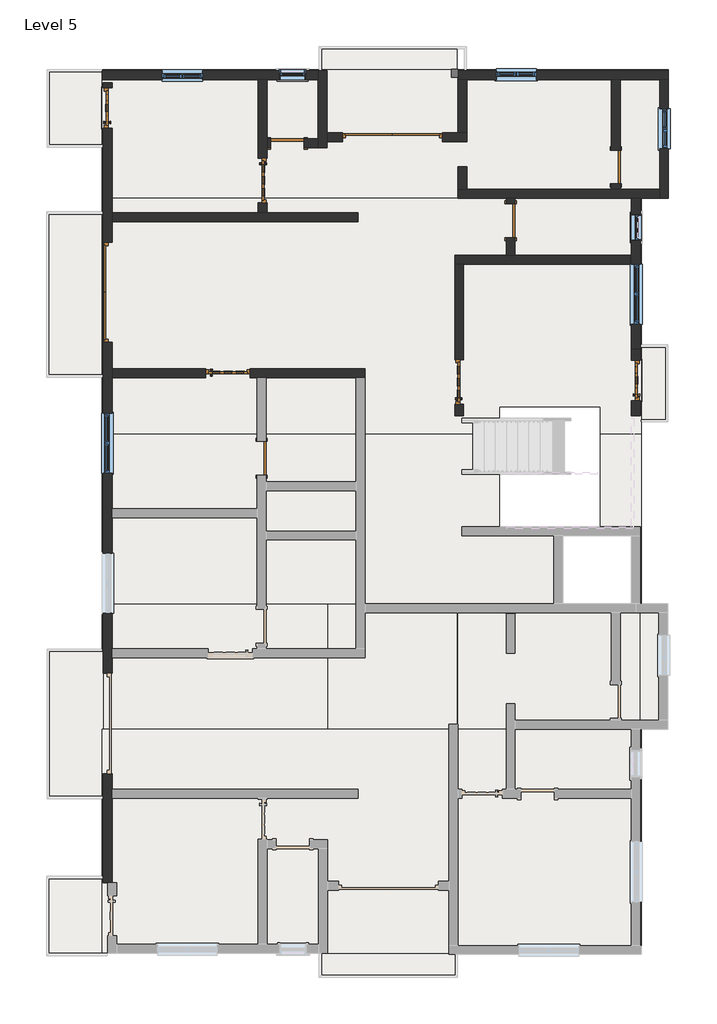
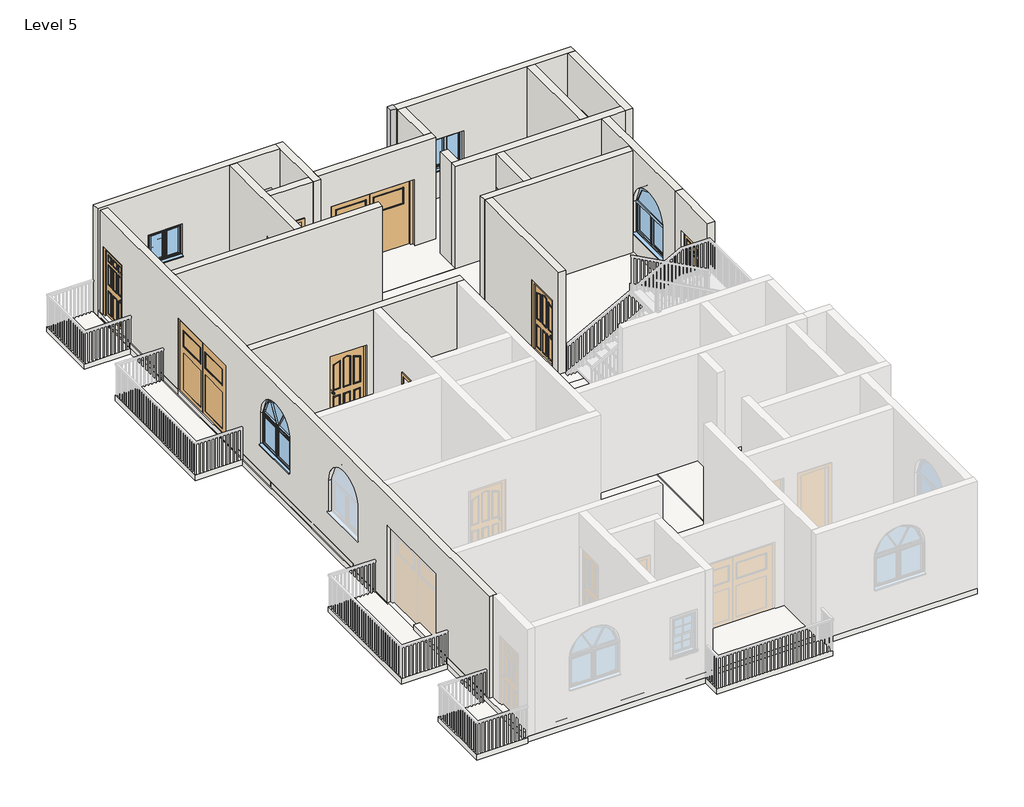
# One storey, part 2 of 7: 19 walls, 11 doors, 10 slabs, 7 windows, 4 roofs, 1 proxy.
# Revit data of these elements (continued)
# Type "Windows_Dbl_w-Glazing_Bars : 910x910mm" (continued)
#   Window Board Extension = 0' - 0.98425"
#   Visual Light Transmittance = 0.9
#   Solar Heat Gain Coefficient = 0.78
#   Rough Width = 2' - 11.82677"
#   Rough Height = 2' - 11.82677"
#   Height = 2' - 11.82677"
#   Width = 2' - 11.82677"
#   Heat Transfer Coefficient (U) = 0.6496 BTU/(h·ft²·°F)
#   Glazing Thickness = 0' - 0.94488"
#   Glazing Bar Thickness = 0' - 0.7874"
#   FrameOffset - External = 0' - 1.9685"
#   Frame Depth = 0' - 2.55906"
#   Default Head Height = 6' - 10.67717"
#   Cill Depth = 0' - 3.44488"
#   Cavity Closer Width = 0' - 1.9685"
#   Cavity Closer Offset from Ext = 0' - 4.03543"
#   Cavity Closer Depth = 0' - 3.34646"
#   Vis - Glazing Bars = yes
#   Vis - Cavity Closers = yes
#   Define Thermal Properties by = 1
#   Material Trim = Window Frame
#   Material Glazing Bars = Window Frame
#   Material Glass = Glass
#   Material Frame = Window Frame
#   Wall Closure = (empty or 0)
# Elements 2, 3 (IfcDoor, "Doors_ExtSgl_5 : 910x2110mm")
#   Phase Created = New Construction
#   Materials on its faces: "Door - Panel", "Door - Handle", "Door - Frame/Mullion", "Door - Glazing"
# Elements 4, 5, 6 (IfcDoor, "Doors_ExtSgl_6 : 1010x2110mm")
#   Phase Created = New Construction
#   Materials on its faces: "Door - Panel", "Door - Handle", "Door - Frame/Mullion", "Door - Glazing"
# Element 7 (IfcDoor, "Doors_Garage_Timber_Side_Hung_Glazing : 2270x2050mm")
#   Phase Created = New Construction
#   Materials on its faces: "Door - Panel", "Door - Frame/Mullion", "Door - Glazing"
# Element 8 (IfcDoor, "Doors_Garage_Timber_Side_Hung_Glazing : 2270x2200mm")
#   Phase Created = New Construction
#   Materials on its faces: "Door - Panel", "Door - Frame/Mullion", "Door - Glazing"
# Elements 9, 10, 11, 12 (IfcDoor, "Single-Flush : 30\" x 80\"")
#   Phase Created = New Construction
#   Materials on its faces: "Door - Frame", "Door - Panel"
# Elements 13, 16 (IfcRoof, "Generic - 12\"")
#   built-in parameter 1001705 = 40.5 (stored number, unit not read)
#   built-in parameter 1001710 = 33615
#   Phase Created = New Construction
#   Materials on its faces: "Default Roof", "Earth"
# Element 14 (IfcRoof, "Generic - 12\"")
#   built-in parameter 1001705 = 40.5 (stored number, unit not read)
#   built-in parameter 1001710 = 33615
#   Phase Created = New Construction
#   Materials on its faces: "Default Roof", "Concrete, Lightweight"
# Element 15 (IfcRoof, "Generic - 12\"")
#   built-in parameter 1001705 = 40.5 (stored number, unit not read)
#   built-in parameter 1001710 = 33615
#   Phase Created = New Construction
#   Materials on its faces: "Default Roof", "Wood - Stained"
# Element 17 (IfcSlab, "Generic - 12\"")
#   Height Offset From Level = 0' - 0"
#   Phase Created = New Construction
#   Materials on its faces: "Default Floor", "Oak Flooring", "Concrete, Lightweight"
# Element 18 (IfcSlab, "Generic - 12\"")
#   Height Offset From Level = 0' - 0"
#   Phase Created = New Construction
#   Materials on its faces: "Default Floor", "Earth", "Concrete, Lightweight", "Wood - Stained"
# Element 19 (IfcSlab, "Generic - 12\"")
#   Height Offset From Level = 0' - 0"
#   Phase Created = New Construction
#   Materials on its faces: "Default Floor", "Earth"
# Element 20 (IfcSlab, "Generic - 12\"")
#   Height Offset From Level = 0' - 0"
#   Phase Created = New Construction
#   Materials on its faces: "Default Floor", "Cherry", "Brick, Soldier Course", "mm"
# Elements 21, 22, 23, 24, 25 (IfcSlab, "Generic - 12\"")
#   Height Offset From Level = 0' - 0"
#   Phase Created = New Construction
#   Materials on its faces: "Default Floor"
# Element 26 (IfcSlab, "Generic - 12\"")
#   Height Offset From Level = 0' - 0"
#   Phase Created = New Construction
#   Materials on its faces: "Default Floor", "Concrete, Lightweight", "Earth"
# Elements 27, 31 (IfcWall, "Generic - 9\" w")
#   Top Offset = 0' - 0"
#   Base Offset = 0' - 0"
#   wall height = 10' - 0"
#   Phase Created = New Construction
#   Base Constraint = Level 5
#   Top Constraint = Level 6
#   Materials on its faces: "Default Wall", "Earth"
# Element 28 (IfcWall, "Generic - 9\" w")
#   Top Offset = 0' - 0"
#   Base Offset = 0' - 0"
#   wall height = 10' - 0"
#   Phase Created = New Construction
#   Base Constraint = Level 5
#   Top Constraint = Level 6
#   Materials on its faces: "Default Wall", "Wood - Stained"
# Element 29 (IfcWall, "Generic - 9\" w")
#   Top Offset = 0' - 0"
#   Base Offset = 0' - 0"
#   wall height = 10' - 0"
#   Phase Created = New Construction
#   Base Constraint = Level 5
#   Top Constraint = Level 6
#   Materials on its faces: "Default Wall", "Grass"
# Element 30 (IfcWall, "Generic - 9\" w")
#   Top Offset = 0' - 0"
#   Base Offset = 0' - 0"
#   wall height = 10' - 0"
#   Phase Created = New Construction
#   Base Constraint = Level 5
#   Top Constraint = Level 6
#   Materials on its faces: "Default Wall", "mm"
# Elements 32, 33, 35, 37, 38, 40, 41, 42, 43, 44, 45 (IfcWall, "Generic -4.5\" p")
#   Top Offset = 0' - 0"
#   Base Offset = 0' - 0"
#   wall height = 10' - 0"
#   Phase Created = New Construction
#   Base Constraint = Level 5
#   Top Constraint = Level 6
#   Materials on its faces: "Default Wall"
# Elements 34, 39 (IfcWall, "Generic -4.5\" p")
#   Top Offset = 0' - 0"
#   Base Offset = 0' - 0"
#   wall height = 10' - 0"
#   Phase Created = New Construction
#   Base Constraint = Level 5
#   Top Constraint = Level 6
#   Materials on its faces: "Default Wall", "Earth"
# Element 36 (IfcWall, "Generic -4.5\" p")
#   Top Offset = 0' - 0"
#   Base Offset = 0' - 0"
#   wall height = 10' - 0"
#   Phase Created = New Construction
#   Base Constraint = Level 5
#   Top Constraint = Level 6
#   Materials on its faces: "Default Wall", "Oak Flooring"
# Element 46 (IfcWindow, "Window-Double-Hung : 24\" x 42\"")
#   Mark = "60"
#   Window Inset = 0' - 0"
#   Interior Wall Closure = 0' - 1 1/2"
#   Frame Extension = 0' - 1 1/4"
#   Exterior Wall Closure = 0' - 0 1/2"
#   Interior Trim Visibility = yes
#   Indicator Visibility = yes
#   Exterior Trim Visibility = yes
#   Phase Created = New Construction
#   Materials on its faces: "Wood - Stained", "Glass", "Clad - White"
# Element 47 (IfcWindow, "Window-Double-Hung : 24\" x 42\"")
#   Mark = "66"
#   Window Inset = 0' - 0"
#   Interior Wall Closure = 0' - 1 1/2"
#   Frame Extension = 0' - 1 1/4"
#   Exterior Wall Closure = 0' - 0 1/2"
#   Interior Trim Visibility = yes
#   Indicator Visibility = yes
#   Exterior Trim Visibility = yes
#   Phase Created = New Construction
#   Materials on its faces: "Wood - Stained", "Glass", "Clad - White"
# Element 48 (IfcWindow, "Windows_Arched : 1360x910mm")
#   Mark = "56"
#   Phase Created = New Construction
#   Materials on its faces: "Window Frame", "Glass"
# Element 49 (IfcWindow, "Windows_Arched : 1360x910mm")
#   Mark = "67"
#   Phase Created = New Construction
#   Materials on its faces: "Window Frame", "Glass"
# Element 50 (IfcWindow, "Windows_Dbl_w-Glazing_Bars : 910x910mm")
#   Mark = "63"
#   Phase Created = New Construction
#   Materials on its faces: "Window Frame", "Glass"
# Element 51 (IfcWindow, "Windows_Dbl_w-Glazing_Bars : 910x910mm")
#   Mark = "64"
#   Phase Created = New Construction
#   Materials on its faces: "Window Frame", "Glass"
# Element 52 (IfcWindow, "Windows_Dbl_w-Glazing_Bars : 910x910mm")
#   Mark = "65"
#   Phase Created = New Construction
#   Materials on its faces: "Window Frame", "Glass"
# Materials
#   "Door - Glazing": colour RGB 0 0 255, transparency 0.75
#   "Door - Panel": class "Wood", colour RGB 210 159 95, transparency 0, Cost = 0
#   "Door - Frame/Mullion": class "Wood", colour RGB 212 179 113, transparency 0
#   "Door - Handle": colour RGB 0 0 0, transparency 0
#   "Door - Frame": colour RGB 118 70 51, transparency 0, Cost = 0
#   "Wood - Stained": class "Wood", colour RGB 224 178 126, transparency 0, Cost = 0
#   "Clad - White": class "Wood", colour RGB 242 242 238, transparency 0, Cost = 0
#   "Glass": class "Glass", colour RGB 0 128 192, transparency 0.75, Description = "Soda Lime Glass", Cost = 0
#   "Window Frame": colour RGB 249 249 249, transparency 0
#   "Default Roof": colour RGB 88 101 114, transparency 0, Cost = 0
#   "Earth": class "Generic", colour RGB 97 75 62, transparency 0, Description = "Soil", Cost = 0
#   "Concrete, Lightweight": class "Concrete", colour RGB 142 141 140, transparency 0, Description = "Lightweight concrete", Cost = 0
#   "Default Floor": colour RGB 128 128 128, transparency 0, Cost = 0
#   "Oak Flooring": class "Wood", colour RGB 216 169 114, transparency 0, Description = "Quercus Rubra", Cost = 0
#   "Cherry": class "Wood", colour RGB 226 177 128, transparency 0, Description = "Prunus Serotina", Cost = 0
#   "Brick, Soldier Course": class "Masonry", colour RGB 170 98 104, transparency 0, Description = "Common brick soldier coursed", Cost = 0
#   "mm": class "Generic", colour RGB 128 64 0, transparency 0.5, Cost = 0
#   "Default Wall": colour RGB 128 128 128, transparency 0, Cost = 0
#   "Grass": class "Generic", colour RGB 104 137 66, transparency 0, Description = "Physical material.", Cost = 0
